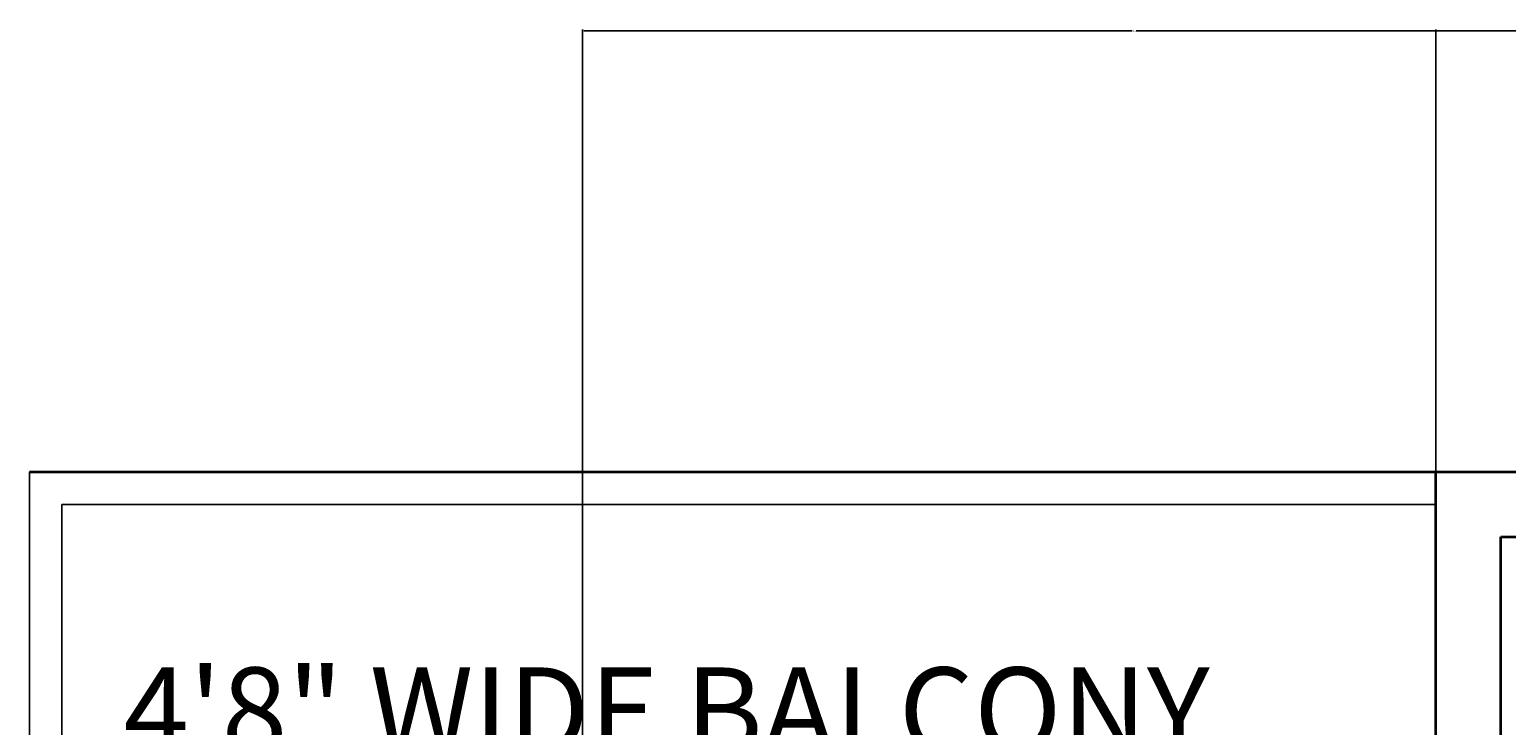
# Model space of a CAD drawing. Units: feet. Extents: x 5816 to 6644, y 25475 to 26788.
# Tile 14 of 23: x 5877 to 6082, y 26691 to 26788. Entities that reach past the tile are written whole.
import ezdxf

# ---------------------------------------------------------------- set-up
doc = ezdxf.new("R2010")
doc.units = ezdxf.units.FT
for name, color, linetype, lineweight in [('A-ANNO-DIMS', 2, 'Continuous', 13), ('A-AREA-IDEN', 7, 'Continuous', 18), ('A-FLOR-RAIL', 8, 'Continuous', 25), ('A-WALL', 7, 'Continuous', 35)]:
    doc.layers.add(name, color=color, linetype=linetype, lineweight=lineweight)
doc.styles.get("Standard").update_dxf_attribs({"font": 'arial.ttf'})
doc.dimstyles.get("Standard").update_dxf_attribs({"dimtxt": 0.18, "dimasz": 0.18, "dimexe": 0.18, "dimexo": 0.0625, "dimgap": 0.09, "dimtad": 0, "dimtih": 1, "dimtoh": 1, "dimdec": 4, "dimzin": 0, "dimdsep": 46, "dimtxsty": 'Standard', "dimcen": 0.09, "dimadec": 0, "dimazin": 0, "dimtfac": 1, "dimtdec": 4, "dimtofl": 0, "dimtmove": 0, "dimatfit": 3, "dimfxl": 1, "dimtolj": 1, "dimtzin": 0, "dimarcsym": 0})

# ---------------------------------------------------------------- blocks, each defined once
blk = doc.blocks.new('RAIL-BALCONY-CORNER')
for p, q in [((0, 0), (0, -65)), ((0, 0), (195, 0)), ((4.5, -4.5), (4.5, -65)), ((4.5, -4.5), (195, -4.5))]:
    blk.add_line(p, q)
blk = doc.blocks.new('*D58')
at = {"layer": 'A-ANNO-DIMS', "color": 0, "lineweight": -2, "transparency": 16777216}
for p, q in [((5953.98, 26168.65), (5953.98, 26787.91)), ((5954.16, 26787.73), (6030.2, 26787.73)), ((6106.8, 26787.73), (6030.76, 26787.73)), ((6106.98, 26168.71), (6106.98, 26787.91))]:
    blk.add_line(p, q, dxfattribs=at)
at = {"layer": 'A-ANNO-DIMS', "color": 0, "transparency": 16777216}
for points in [[(5954.16, 26787.76), (5954.16, 26787.7), (5953.98, 26787.73)], [(6106.8, 26787.76), (6106.8, 26787.7), (6106.98, 26787.73)]]:
    blk.add_solid(points, dxfattribs=at)
at = {"layer": 'Defpoints', "color": 0, "transparency": 16777216}
for p in [(6106.98, 26787.73), (5953.98, 26168.58), (6106.98, 26168.65)]:
    blk.add_point(p, dxfattribs=at)
at = {"layer": 'A-ANNO-DIMS', "color": 0, "transparency": 16777216, "insert": (6030.48, 26787.73), "char_height": 0.18, "attachment_point": 5}
blk.add_mtext('\\A1;153', dxfattribs=at)
blk = doc.blocks.new('*D63')
at = {"layer": 'A-ANNO-DIMS', "color": 0, "lineweight": -2, "transparency": 16777216}
for p, q in [((6072.31, 26726.65), (6072.31, 26787.91)), ((6072.49, 26787.73), (6100.95, 26787.73)), ((6130.2, 26787.73), (6101.74, 26787.73)), ((6130.38, 26726.65), (6130.38, 26787.91))]:
    blk.add_line(p, q, dxfattribs=at)
at = {"layer": 'A-ANNO-DIMS', "color": 0, "transparency": 16777216}
for points in [[(6072.49, 26787.76), (6072.49, 26787.7), (6072.31, 26787.73)], [(6130.2, 26787.76), (6130.2, 26787.7), (6130.38, 26787.73)]]:
    blk.add_solid(points, dxfattribs=at)
at = {"layer": 'Defpoints', "color": 0, "transparency": 16777216}
for p in [(6130.38, 26787.73), (6072.31, 26726.58), (6130.38, 26726.58)]:
    blk.add_point(p, dxfattribs=at)
at = {"layer": 'A-ANNO-DIMS', "color": 0, "transparency": 16777216, "insert": (6101.35, 26787.73), "char_height": 0.18, "attachment_point": 5}
blk.add_mtext('\\A1;58.07', dxfattribs=at)

msp = doc.modelspace()

# ---------------------------------------------------------------- linework, layer by layer
at = {"layer": 'A-WALL'}
for p, q in [((5877.3119, 26726.5846), (6279.7398, 26726.5846)), ((6072.3119, 26661.5846), (6072.3119, 26726.5846)), ((6081.3119, 26661.5846), (6081.3119, 26717.5846)), ((6081.3119, 26717.5846), (6225.3119, 26717.5846))]:
    msp.add_line(p, q, dxfattribs=at)

# ---------------------------------------------------------------- block references
at = {"layer": 'A-FLOR-RAIL'}
msp.add_blockref('RAIL-BALCONY-CORNER', (5877.3119, 26726.5846), dxfattribs=at)

# ---------------------------------------------------------------- texts
at = {"layer": 'A-AREA-IDEN'}
msp.add_text('4\'8" WIDE BALCONY', height=12, dxfattribs=at).set_placement((5890.3368, 26687.4804))

# ---------------------------------------------------------------- dimensions: what is measured, and where the dimension line sits
at = {"layer": 'A-ANNO-DIMS'}
for base, p1, p2, override, picture, middle in [((6106.9781, 26787.7346), (5953.9781, 26168.5846), (6106.9781, 26168.6509), {"dimdec": 0, "dimlfac": 1, "dimrnd": 0, "dimzin": 0, "dimdsep": 46, "dimlunit": 2}, '*D58', (6030.4781, 26787.7346)), ((6130.3809, 26787.7346), (6072.3119, 26726.5846), (6130.3809, 26726.5846), {"dimdec": 2, "dimlfac": 1, "dimrnd": 0, "dimzin": 0, "dimdsep": 46, "dimlunit": 2}, '*D63', (6101.3464, 26787.7346))]:
    dim = msp.add_linear_dim(base=base, p1=p1, p2=p2, dimstyle='Standard', override=override, dxfattribs=at)
    dim.commit()
    dim.dimension.update_dxf_attribs({"geometry": picture, "text_midpoint": middle})

doc.saveas('drawing.dxf')
